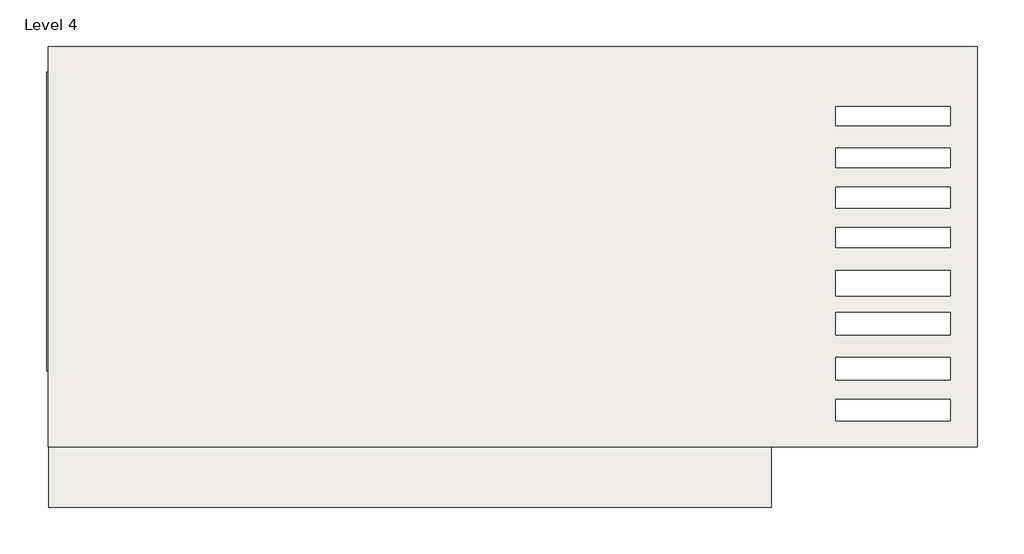
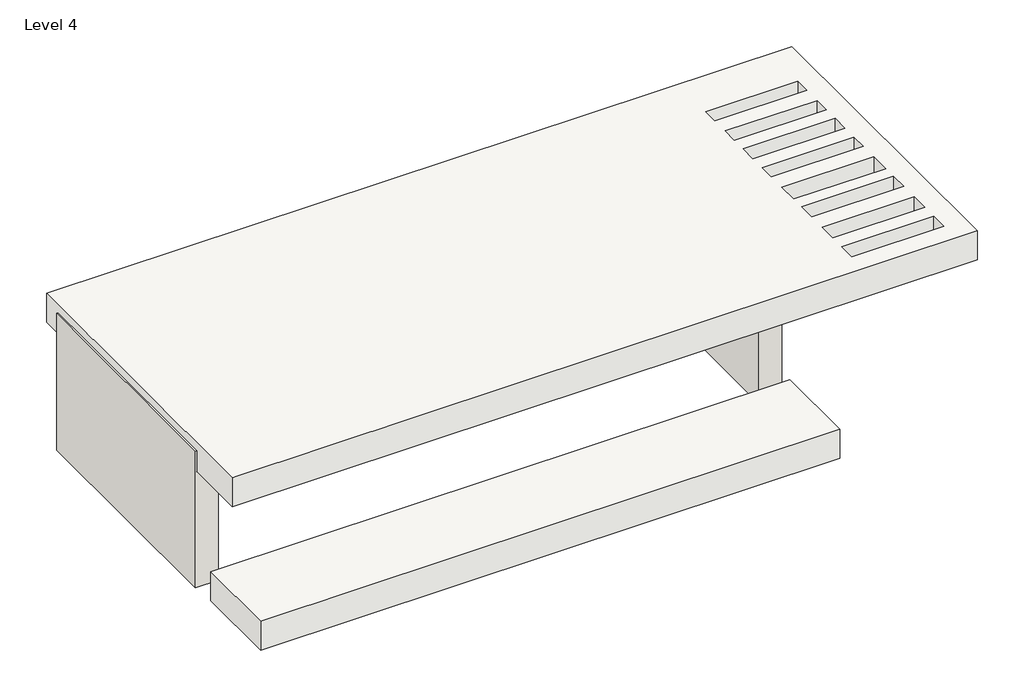
# One storey: 2 roofs, 2 walls.
"""IFC4 building model written with IfcOpenShell, lengths in millimetres."""

from ifc_helpers import new_model, si_unit, frame, origin, place, context, project, spatial, polyline, outline, extrude, faceted_brep, element, save

model = new_model("IFC4")

# Units and contexts
model_context = context("Model", 3, world=origin())
ifc_project = project(units=[si_unit("LENGTHUNIT", "METRE", prefix="MILLI")], contexts=[model_context])

# Site, building, storey
site = spatial("IfcSite", under=ifc_project)
building = spatial("IfcBuilding", under=site)
storey = spatial("IfcBuildingStorey", under=building, Name="Level 4", Elevation=10972.8)

# Roofs
placement = place(None, origin())
element("IfcRoof", 1, ObjectType="Generic - 12\"", at=placement, inside=storey, context=model_context, shape_type="SweptSolid", body=[
    extrude(outline(polyline([(-13805.7728698, -2888.2259649), (-8039.9728698, -2888.2259649), (-8039.9728698, -3751.8259649), (-13805.7728698, -3751.8259649), (-13805.7728698, -2888.2259649)])), frame((0.0, 0.0, 9753.6), z_axis=(0.0, 0.0, 1.0), x_axis=(1.0, 0.0, 0.0)), (0.0, 0.0, 1.0), 304.8),
])
element("IfcRoof", 2, ObjectType="Generic - 12\"", at=placement, inside=storey, context=model_context, shape_type="SweptSolid", body=[
    extrude(outline(polyline([(-13810.1555193, -68.8259649), (-6393.3555193, -68.8259649), (-6393.3555193, -3269.2259649), (-13810.1555193, -3269.2259649), (-13810.1555193, -68.8259649)]), holes=[polyline([(-6610.0329588, -700.8278755), (-6610.0329588, -548.4278755), (-7524.4329588, -548.4278755), (-7524.4329588, -700.8278755), (-6610.0329588, -700.8278755)]), polyline([(-6610.0329588, -1037.8842765), (-6610.0329588, -881.0246059), (-7524.4329588, -881.0246059), (-7524.4329588, -1037.8842765), (-6610.0329588, -1037.8842765)]), polyline([(-6610.0329588, -1358.4236034), (-6610.0329588, -1191.3339543), (-7524.4329588, -1191.3339543), (-7524.4329588, -1358.4236034), (-6610.0329588, -1358.4236034)]), polyline([(-6610.0329588, -1675.5529375), (-6610.0329588, -1515.283274), (-7524.4329588, -1515.283274), (-7524.4329588, -1675.5529375), (-6610.0329588, -1675.5529375)]), polyline([(-6610.0329588, -2060.4303043), (-6610.0329588, -1857.4931054), (-7524.4329588, -1857.4931054), (-7524.4329588, -2060.4303043), (-6610.0329588, -2060.4303043)]), polyline([(-6610.0329588, -2371.6006759), (-6610.0329588, -2195.7217702), (-7524.4329588, -2195.7217702), (-7524.4329588, -2371.6006759), (-6610.0329588, -2371.6006759)]), polyline([(-6610.0329588, -2732.3779183), (-6610.0329588, -2551.9892971), (-7524.4329588, -2551.9892971), (-7524.4329588, -2732.3779183), (-6610.0329588, -2732.3779183)]), polyline([(-6610.0329588, -3061.587152), (-6610.0329588, -2888.2259649), (-7524.4329588, -2888.2259649), (-7524.4329588, -3061.587152), (-6610.0329588, -3061.587152)])]), frame((0.0, 0.0, 10972.8), z_axis=(0.0, 0.0, 1.0), x_axis=(1.0, 0.0, 0.0)), (0.0, 0.0, 1.0), 304.8),
])

# Walls
element("IfcWall", 3, ObjectType="Generic - 8\" - Filled", at=placement, inside=storey, context=model_context, shape_type="Brep", body=[
    faceted_brep([(-13824.8228698, -272.0259649, 9753.6), (-13824.8228698, -2659.6259649, 9753.6), (-13824.8228698, -2659.6259649, 11194.4859918), (-13824.8228698, -272.0259649, 11194.4859918), (-13596.2228698, -272.0259649, 9753.6), (-13596.2228698, -272.0259649, 10972.8), (-13596.2228698, -2659.6259649, 10972.8), (-13596.2228698, -2659.6259649, 9753.6), (-13626.0055193, -272.0259649, 9753.6), (-13810.1555193, -272.0259649, 11194.4859918), (-13810.1555193, -272.0259649, 10972.8), (-13810.1555193, -2659.6259649, 10972.8), (-13810.1555193, -2659.6259649, 11194.4859918)], [[[0, 1, 2, 3]], [[4, 5, 6, 7]], [[1, 0, 8, 4, 7]], [[0, 3, 9, 10, 5, 4, 8]], [[2, 1, 7, 6, 11, 12]], [[3, 2, 12, 9]], [[9, 12, 11, 10]], [[11, 6, 5, 10]]]),
])
element("IfcWall", 4, ObjectType="Generic - 8\" - Filled", at=placement, inside=storey, context=model_context, shape_type="Brep", body=[
    faceted_brep([(-8217.7728698, -272.0259649, 9731.3133194), (-8217.7728698, -2659.6259649, 9731.3133194), (-8217.7728698, -2659.6259649, 10972.8), (-8217.7728698, -272.0259649, 10972.8), (-7989.1728698, -272.0259649, 9731.3133194), (-7989.1728698, -272.0259649, 10972.8), (-7989.1728698, -2659.6259649, 10972.8), (-7989.1728698, -2659.6259649, 9753.6), (-7989.1728698, -2659.6259649, 9731.3133194)], [[[0, 1, 2, 3]], [[4, 5, 6, 7, 8]], [[1, 0, 4, 8]], [[0, 3, 5, 4]], [[2, 1, 8, 7, 6]], [[3, 2, 6, 5]]]),
])

save(model, "model.ifc")

# Revit data of these elements
# Type "Generic - 12\""
#   Assembly Code = "B1020"
#   Layers, outside or top first: 1' - 0" no material (function 1)
# Type "Generic - 8\" - Filled"
#   Assembly Code = "B2010"
#   Layers, outside or top first: 0' - 9" no material (function 1)
# Element 1 (IfcRoof, "Generic - 12\"")
#   built-in parameter 1001705 = 33 (stored number, unit not read)
#   built-in parameter 1001701 = -4 (stored number, unit not read)
#   built-in parameter 1001710 = 33615
#   Phase Created = New Construction
#   Materials on its faces: "Default Roof"
# Element 2 (IfcRoof, "Generic - 12\"")
#   built-in parameter 1001705 = 37 (stored number, unit not read)
#   built-in parameter 1001710 = 33615
#   Phase Created = New Construction
#   Materials on its faces: "Default Roof"
# Element 3 (IfcWall, "Generic - 8\" - Filled")
#   built-in parameter 1001111 = -4' - 0"
#   Top Offset = 0' - 0"
#   Base Offset = -4' - 0"
#   Unconnected Height = 4' - 8.72779"
#   wall height = 4' - 8.72779"
#   Phase Created = New Construction
#   Base Constraint = Level 4
#   Materials on its faces: "Default Wall"
# Element 4 (IfcWall, "Generic - 8\" - Filled")
#   built-in parameter 1001111 = -4' - 0.87743"
#   Top Offset = 0' - 0"
#   Base Offset = -4' - 0.87743"
#   Unconnected Height = 4' - 9.60522"
#   wall height = 4' - 9.60522"
#   Phase Created = New Construction
#   Base Constraint = Level 4
#   Materials on its faces: "Default Wall"
# Materials
#   "Default Roof": colour RGB 88 101 114, transparency 0
#   "Default Wall": colour RGB 128 128 128, transparency 0
